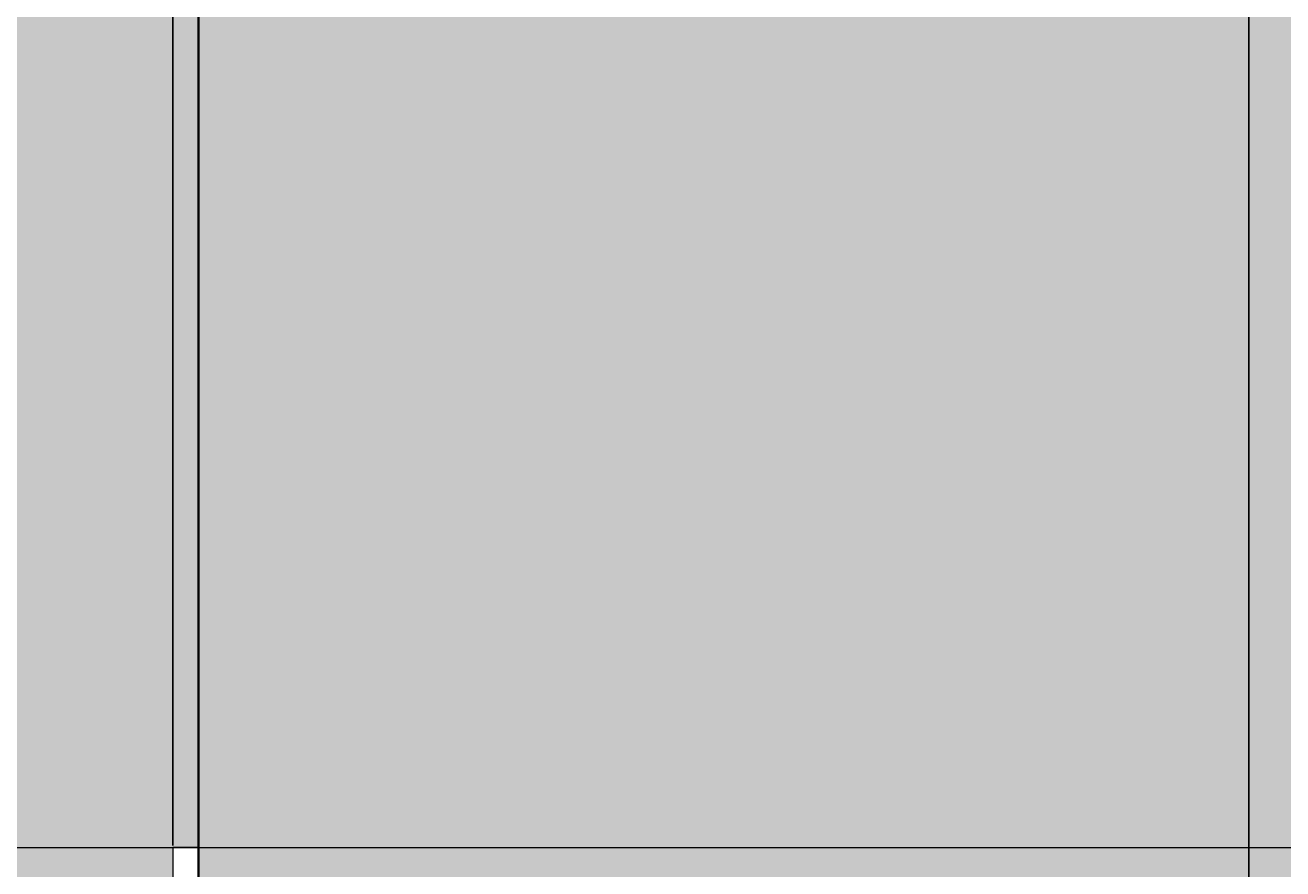
# Model space of a CAD drawing. Units: feet. Extents: x 2695 to 2912, y 795 to 1139.
# Tile 55 of 83: x 2806 to 2843, y 971 to 996. Entities that reach past the tile are written whole.
import ezdxf

# ---------------------------------------------------------------- set-up
doc = ezdxf.new("R2010")
doc.units = ezdxf.units.FT
for name, color, linetype, lineweight in [('A-ANNO-DIMS', 2, 'Continuous', 18), ('A-ELEV-PATT', 252, 'Continuous', 13), ('A-ELEV-RAIL', 8, 'Continuous', 18), ('A-GLAZ', 4, 'Continuous', 25), ('A-GLAZ-PATT', 254, 'Continuous', 13)]:
    doc.layers.add(name, color=color, linetype=linetype, lineweight=lineweight)
doc.styles.get("Standard").update_dxf_attribs({"font": 'arial.ttf'})
doc.dimstyles.get("Standard").update_dxf_attribs({"dimtxt": 0.18, "dimasz": 0.18, "dimexe": 0.18, "dimexo": 0.0625, "dimgap": 0.09, "dimtad": 0, "dimtih": 1, "dimtoh": 1, "dimdec": 1, "dimzin": 0, "dimdsep": 46, "dimlunit": 3, "dimtxsty": 'Standard', "dimcen": 0.09, "dimadec": 0, "dimazin": 0, "dimtfac": 1, "dimtdec": 1, "dimtofl": 0, "dimtmove": 0, "dimatfit": 3, "dimfxl": 1, "dimtolj": 1, "dimtzin": 0, "dimarcsym": 0})

# ---------------------------------------------------------------- blocks, each defined once
blk = doc.blocks.new('*D49')
at = {"layer": 'A-ANNO-DIMS', "color": 0, "lineweight": -2, "transparency": 16777216}
for p, q in [((2772.522, 972.03), (2772.522, 1138.886)), ((2772.702, 1138.706), (2790.888, 1138.706)), ((2809.861, 1138.706), (2791.674, 1138.706)), ((2810.041, 972.03), (2810.041, 1138.886))]:
    blk.add_line(p, q, dxfattribs=at)
at = {"layer": 'A-ANNO-DIMS', "color": 0, "transparency": 16777216}
for points in [[(2772.702, 1138.736), (2772.702, 1138.676), (2772.522, 1138.706)], [(2809.861, 1138.736), (2809.861, 1138.676), (2810.041, 1138.706)]]:
    blk.add_solid(points, dxfattribs=at)
at = {"layer": 'Defpoints', "color": 0, "transparency": 16777216}
for p in [(2810.041, 1138.706), (2772.522, 971.967), (2810.041, 971.967)]:
    blk.add_point(p, dxfattribs=at)
at = {"layer": 'A-ANNO-DIMS', "color": 0, "transparency": 16777216, "insert": (2791.281, 1138.706), "char_height": 0.18, "attachment_point": 5}
blk.add_mtext('\\A1;37.52', dxfattribs=at)
blk = doc.blocks.new('*D50')
at = {"layer": 'A-ANNO-DIMS', "color": 0, "lineweight": -2, "transparency": 16777216}
for p, q in [((2810.041, 972.03), (2810.041, 1138.886)), ((2810.221, 1138.706), (2848.721, 1138.706)), ((2888.008, 1138.706), (2849.508, 1138.706)), ((2888.188, 972.03), (2888.188, 1138.886))]:
    blk.add_line(p, q, dxfattribs=at)
at = {"layer": 'A-ANNO-DIMS', "color": 0, "transparency": 16777216}
for points in [[(2810.221, 1138.736), (2810.221, 1138.676), (2810.041, 1138.706)], [(2888.008, 1138.736), (2888.008, 1138.676), (2888.188, 1138.706)]]:
    blk.add_solid(points, dxfattribs=at)
at = {"layer": 'Defpoints', "color": 0, "transparency": 16777216}
for p in [(2888.188, 1138.706), (2810.041, 971.967), (2888.188, 971.967)]:
    blk.add_point(p, dxfattribs=at)
at = {"layer": 'A-ANNO-DIMS', "color": 0, "transparency": 16777216, "insert": (2849.114, 1138.706), "char_height": 0.18, "attachment_point": 5}
blk.add_mtext('\\A1;78.15', dxfattribs=at)

msp = doc.modelspace()

# ---------------------------------------------------------------- hatches: boundary and pattern name
at = {"layer": 'A-ELEV-PATT'}
h = msp.add_hatch(color=256, dxfattribs=at)
h.set_gradient(color2=(0, 0, 0), tint=1)
h.paths.add_polyline_path([(2772.5216, 971.9673), (2770.6361, 971.9673), (2770.6361, 970.7156), (2772.5216, 970.7156)])
h.paths.add_polyline_path([(2773.2702, 971.9673), (2772.5216, 971.9673), (2772.5216, 970.7156), (2773.2702, 970.7156)])
h.paths.add_polyline_path([(2778.0341, 971.9673), (2773.2702, 971.9673), (2773.2702, 970.7156), (2778.0341, 970.7156)])
h.paths.add_polyline_path([(2780.0341, 971.9673), (2778.0341, 971.9673), (2778.0341, 970.7156), (2780.0341, 970.7156)])
h.paths.add_polyline_path([(2841.575, 971.9673), (2780.0341, 971.9673), (2780.0341, 970.7156), (2841.575, 970.7156)])
h.paths.add_polyline_path([(2843.575, 971.9673), (2841.575, 971.9673), (2841.575, 970.7156), (2843.575, 970.7156)])
h.paths.add_polyline_path([(2888.1882, 971.9673), (2843.575, 971.9673), (2843.575, 970.7156), (2888.1882, 970.7156)])
h.paths.add_polyline_path([(2888.9368, 971.9673), (2888.1882, 971.9673), (2888.1882, 970.7156), (2888.9368, 970.7156)], flags=17)
h.paths.add_polyline_path([(2890.6361, 971.9673), (2888.9368, 971.9673), (2888.9368, 970.7156), (2890.6361, 970.7156)])
h.paths.add_polyline_path([(2888.9368, 971.9673), (2888.1882, 971.9673), (2888.1882, 964.8267), (2888.9368, 964.8267)])
h.paths.add_polyline_path([(2888.9368, 964.8267), (2888.1882, 964.8267), (2888.1882, 964.1328), (2888.9368, 964.1328)])
h.paths.add_polyline_path([(2890.6361, 964.8267), (2888.9368, 964.8267), (2888.9368, 964.1328), (2890.6361, 964.1328)])
h.paths.add_polyline_path([(2888.1882, 964.8267), (2770.6361, 964.8267), (2770.6361, 964.1328), (2888.1882, 964.1328)])
h.paths.add_polyline_path([(2888.9368, 964.1328), (2888.1882, 964.1328), (2888.1882, 936.9306), (2888.9368, 936.9306)])
h.paths.add_polyline_path([(2890.6361, 956.614), (2888.9368, 956.614), (2888.9368, 955.9202), (2890.6361, 955.9202)])
h.paths.add_polyline_path([(2888.1882, 956.614), (2770.6361, 956.614), (2770.6361, 955.9202), (2888.1882, 955.9202)])
h.paths.add_polyline_path([(2890.6361, 949.2892), (2888.9368, 949.2892), (2888.9368, 948.5954), (2890.6361, 948.5954)])
h.paths.add_polyline_path([(2888.1882, 949.2892), (2770.6361, 949.2892), (2770.6361, 948.5954), (2888.1882, 948.5954)])
h.paths.add_polyline_path([(2890.6361, 941.3507), (2888.9368, 941.3507), (2888.9368, 940.6569), (2890.6361, 940.6569)])
h.paths.add_polyline_path([(2888.1882, 941.3507), (2770.6361, 941.3507), (2770.6361, 940.6569), (2888.1882, 940.6569)])
h.paths.add_polyline_path([(2773.2702, 970.7156), (2772.5216, 970.7156), (2772.5216, 964.8267), (2773.2702, 964.8267)])
h.paths.add_polyline_path([(2773.2702, 964.1328), (2772.5216, 964.1328), (2772.5216, 956.614), (2773.2702, 956.614)])
h.paths.add_polyline_path([(2773.2702, 955.9202), (2772.5216, 955.9202), (2772.5216, 936.9306), (2773.2702, 936.9306)])
h.paths.add_polyline_path([(2810.7893, 970.7156), (2810.0407, 970.7156), (2810.0407, 964.8267), (2810.7893, 964.8267)], flags=17)
h.paths.add_polyline_path([(2810.7893, 964.1328), (2810.0407, 964.1328), (2810.0407, 956.614), (2810.7893, 956.614)], flags=17)
h.paths.add_polyline_path([(2810.7893, 955.9202), (2810.0407, 955.9202), (2810.0407, 949.2892), (2810.7893, 949.2892)], flags=17)
h.paths.add_polyline_path([(2810.7893, 971.9673), (2810.0407, 971.9673), (2810.0407, 941.3507), (2810.7893, 941.3507)])
h.paths.add_polyline_path([(2810.7893, 940.6569), (2810.0407, 940.6569), (2810.0407, 936.9306), (2810.7893, 936.9306)])
h.paths.add_polyline_path([(2780.0341, 1018.8235), (2841.575, 1018.8235), (2841.575, 971.9673), (2843.575, 971.9673), (2843.575, 1020.8235), (2778.0341, 1020.8235), (2778.0341, 971.9673), (2780.0341, 971.9673)])
h.paths.add_polyline_path([(2780.0341, 970.7156), (2778.0341, 970.7156), (2778.0341, 964.8267), (2780.0341, 964.8267)])
h.paths.add_polyline_path([(2780.0341, 964.1328), (2778.0341, 964.1328), (2778.0341, 956.614), (2780.0341, 956.614)])
h.paths.add_polyline_path([(2780.0341, 955.9202), (2778.0341, 955.9202), (2778.0341, 949.2892), (2780.0341, 949.2892)])
h.paths.add_polyline_path([(2780.0341, 948.5954), (2778.0341, 948.5954), (2778.0341, 941.3507), (2780.0341, 941.3507)])
h.paths.add_polyline_path([(2780.0341, 940.6569), (2778.0341, 940.6569), (2778.0341, 936.9306), (2780.0341, 936.9306)])
h.paths.add_polyline_path([(2843.575, 940.6569), (2841.575, 940.6569), (2841.575, 936.9306), (2843.575, 936.9306)])
h.paths.add_polyline_path([(2843.575, 948.5954), (2841.575, 948.5954), (2841.575, 941.3507), (2843.575, 941.3507)])
h.paths.add_polyline_path([(2843.575, 970.7156), (2841.575, 970.7156), (2841.575, 964.8267), (2843.575, 964.8267)])
h.paths.add_polyline_path([(2843.575, 964.1328), (2841.575, 964.1328), (2841.575, 956.614), (2843.575, 956.614)])
h.paths.add_polyline_path([(2843.575, 955.9202), (2841.575, 955.9202), (2841.575, 949.2892), (2843.575, 949.2892)])
h.paths.add_polyline_path([(2805.0538, 874.1057), (2803.9681, 874.1057), (2803.9681, 846.2857), (2805.0538, 846.2857)])
h.paths.add_polyline_path([(2758.1515, 902.577), (2724.1893, 902.577), (2724.1893, 874.8571), (2758.1515, 874.8571)])
h.paths.add_polyline_path([(2726.1893, 900.577), (2756.1515, 900.577), (2756.1515, 876.8571), (2726.1893, 876.8571)], flags=16)
h.paths.add_polyline_path([(2740.7302, 900.577), (2741.6105, 900.577), (2741.6105, 876.8571), (2740.7302, 876.8571)], flags=0)
at = {"layer": 'A-GLAZ-PATT'}
h = msp.add_hatch(color=256, dxfattribs=at)
h.set_gradient(color1=(213, 227, 240), color2=(213, 227, 240))
h.paths.add_polyline_path([(2810.8045, 1018.8235), (2780.0341, 1018.8235), (2780.0341, 971.9673), (2810.8045, 971.9673)])
h.paths.add_polyline_path([(2841.575, 1018.8235), (2810.8045, 1018.8235), (2810.8045, 971.9673), (2841.575, 971.9673)])
h.paths.add_polyline_path([(2810.0407, 970.7156), (2780.0341, 970.7156), (2780.0341, 964.8267), (2810.0407, 964.8267)])
h.paths.add_polyline_path([(2841.575, 970.7156), (2810.8045, 970.7156), (2810.8045, 964.8267), (2841.575, 964.8267)])
h.paths.add_polyline_path([(2841.575, 964.1328), (2810.8045, 964.1328), (2810.8045, 956.614), (2841.575, 956.614)])
h.paths.add_polyline_path([(2810.0407, 964.1328), (2780.0341, 964.1328), (2780.0341, 956.614), (2810.0407, 956.614)])
h.paths.add_polyline_path([(2810.0407, 955.9202), (2780.0341, 955.9202), (2780.0341, 949.2892), (2810.0407, 949.2892)])
h.paths.add_polyline_path([(2841.575, 955.9202), (2810.8045, 955.9202), (2810.8045, 949.2892), (2841.575, 949.2892)])
h.paths.add_polyline_path([(2841.575, 948.5954), (2810.8045, 948.5954), (2810.8045, 941.3507), (2841.575, 941.3507)])
h.paths.add_polyline_path([(2810.0407, 948.5954), (2780.0341, 948.5954), (2780.0341, 941.3507), (2810.0407, 941.3507)])
h.paths.add_polyline_path([(2810.0407, 940.6569), (2780.0341, 940.6569), (2780.0341, 936.9306), (2810.0407, 936.9306)])
h.paths.add_polyline_path([(2841.575, 940.6569), (2810.8045, 940.6569), (2810.8045, 936.9306), (2841.575, 936.9306)])

# ---------------------------------------------------------------- linework, layer by layer
at = {"layer": 'A-ELEV-RAIL'}
msp.add_line((2770.6361, 971.9673), (2890.6361, 971.9673), dxfattribs=at)
msp.add_lwpolyline([(2810.7893, 971.9673), (2810.0407, 971.9673), (2810.0407, 936.9306), (2810.7893, 936.9306)], close=True, dxfattribs=at)
at = {"layer": 'A-GLAZ'}
msp.add_line((2810.8045, 1018.8235), (2810.8045, 971.9673), dxfattribs=at)
msp.add_lwpolyline([(2780.0341, 936.9306), (2780.0341, 1018.8235), (2841.575, 1018.8235), (2841.575, 936.9306)], dxfattribs=at)
for points in [[(2810.8045, 1018.8235), (2810.7893, 1018.8235), (2810.7893, 971.9673), (2810.8045, 971.9673)], [(2810.8045, 1018.8235), (2810.7893, 1018.8235), (2810.7893, 936.9306), (2810.8045, 936.9306)], [(2810.8045, 1018.8235), (2810.8045, 1018.8235), (2810.8045, 936.9306), (2810.8045, 936.9306)]]:
    msp.add_lwpolyline(points, close=True, dxfattribs=at)

# ---------------------------------------------------------------- dimensions: what is measured, and where the dimension line sits
at = {"layer": 'A-ANNO-DIMS'}
for base, p1, p2, picture, middle in [((2810.0407, 1138.7056), (2772.5216, 971.9673), (2810.0407, 971.9673), '*D49', (2791.2811, 1138.7056)), ((2888.1882, 1138.7056), (2810.0407, 971.9673), (2888.1882, 971.9673), '*D50', (2849.1144, 1138.7056))]:
    dim = msp.add_linear_dim(base=base, p1=p1, p2=p2, dimstyle='Standard', override={"dimdec": 2, "dimlfac": 1, "dimrnd": 0, "dimzin": 0, "dimdsep": 46, "dimlunit": 2}, dxfattribs=at)
    dim.commit()
    dim.dimension.update_dxf_attribs({"geometry": picture, "text_midpoint": middle})

doc.saveas('drawing.dxf')
